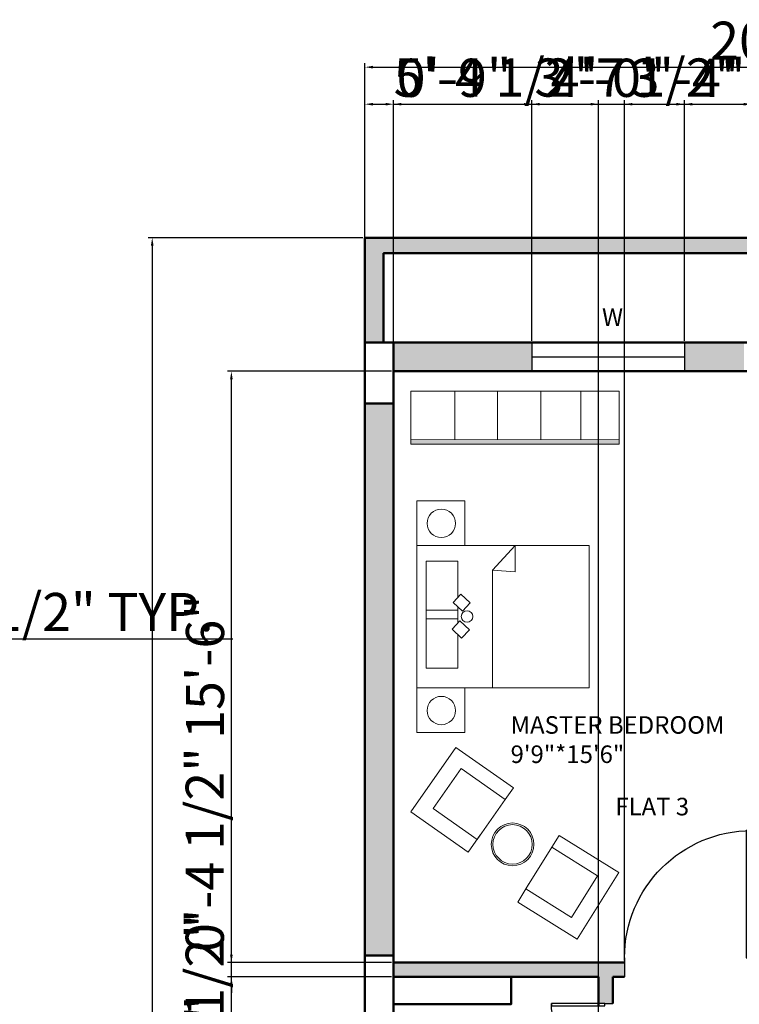
# Model space of a CAD drawing. Units: inches. Extents: x 2063 to 3370, y 2091 to 2971.
# Tile 9 of 14: x 2494 to 2721, y 2623 to 2933. Entities that reach past the tile are written whole.
import ezdxf

# ---------------------------------------------------------------- set-up
doc = ezdxf.new("R2010")
doc.units = ezdxf.units.IN
for name, color, linetype, lineweight in [('A-ANNO-DIMS', 2, 'Continuous', 18), ('A-ANNO-TEXT', 7, 'Continuous', 18), ('A-AREA-IDEN', 3, 'Continuous', 18), ('A-COLS', 7, 'Continuous', 50), ('A-DOOR', 4, 'Continuous', 25), ('A-FURN', 8, 'Continuous', 18), ('A-GLAZ', 131, 'Continuous', 25), ('A-WALL', 7, 'Continuous', 50), ('A-WALL-PATT', 8, 'Continuous', 13)]:
    doc.layers.add(name, color=color, linetype=linetype, lineweight=lineweight)
doc.styles.get("Standard").update_dxf_attribs({"font": 'arial.ttf'})
doc.dimstyles.new('ISO-25', dxfattribs={"dimtxt": 12, "dimasz": 2.5, "dimexe": 1.25, "dimexo": 0.625, "dimtad": 1, "dimdec": 0, "dimlunit": 4, "dimtxsty": 'Standard', "dimcen": 2.5, "dimadec": 0, "dimazin": 0, "dimtfac": 1, "dimtdec": 0, "dimtmove": 0, "dimatfit": 3, "dimfxl": 1, "dimarcsym": 0})

# ---------------------------------------------------------------- blocks, each defined once
blk = doc.blocks.new('*D7')
at = {"layer": 'A-ANNO-DIMS', "color": 0, "lineweight": -2, "transparency": 16777216}
for p, q in [((2602.75, 2865.05), (2602.75, 2919.33)), ((2605.25, 2918.08), (2840.25, 2918.08)), ((2842.75, 2865.05), (2842.75, 2919.33))]:
    blk.add_line(p, q, dxfattribs=at)
at = {"layer": 'A-ANNO-DIMS', "color": 0, "transparency": 16777216}
for points in [[(2605.25, 2918.5), (2605.25, 2917.67), (2602.75, 2918.08)], [(2840.25, 2918.5), (2840.25, 2917.67), (2842.75, 2918.08)]]:
    blk.add_solid(points, dxfattribs=at)
at = {"layer": 'Defpoints', "color": 0, "transparency": 16777216}
for p in [(2842.75, 2918.08), (2602.75, 2864.43), (2842.75, 2864.43)]:
    blk.add_point(p, dxfattribs=at)
at = {"layer": 'A-ANNO-DIMS', "color": 0, "transparency": 16777216, "insert": (2722.75, 2924.84), "char_height": 12, "attachment_point": 5}
blk.add_mtext("20'", dxfattribs=at)
blk = doc.blocks.new('*D8')
at = {"layer": 'A-ANNO-DIMS', "color": 0, "lineweight": -2, "transparency": 16777216}
for p, q in [((2602.12, 2864.43), (2534.59, 2864.43)), ((2535.84, 2861.93), (2535.84, 2146.93)), ((2602.12, 2144.43), (2534.59, 2144.43))]:
    blk.add_line(p, q, dxfattribs=at)
at = {"layer": 'A-ANNO-DIMS', "color": 0, "transparency": 16777216}
for points in [[(2535.42, 2861.93), (2536.25, 2861.93), (2535.84, 2864.43)], [(2535.42, 2146.93), (2536.25, 2146.93), (2535.84, 2144.43)]]:
    blk.add_solid(points, dxfattribs=at)
at = {"layer": 'Defpoints', "color": 0, "transparency": 16777216}
for p in [(2602.75, 2864.43), (2535.84, 2144.43), (2602.75, 2144.43)]:
    blk.add_point(p, dxfattribs=at)
at = {"layer": 'A-ANNO-DIMS', "color": 0, "transparency": 16777216, "insert": (2529.08, 2504.43), "char_height": 12, "attachment_point": 5, "rotation": 90}
blk.add_mtext("60'", dxfattribs=at)
blk = doc.blocks.new('*U2')
for p, q in [((0, 0), (0, -6)), ((40, 0), (40, -6))]:
    blk.add_line(p, q)
blk.add_lwpolyline([(0, 0), (0, 40), (1.75, 40), (1.75, 0)], close=True)
blk.add_arc((0, 0), 40, 0, 90)
blk = doc.blocks.new('BED-DOUBLE')
for p, q in [((23.79, 50.98), (30.96, 58.78)), ((30.96, 58.78), (30.96, 50.54)), ((23.79, 14), (23.79, 50.98)), ((30.96, 50.54), (23.79, 50.98))]:
    blk.add_line(p, q)
for points in [[(0, 58.78), (15.11, 58.78), (15.11, 72.78), (0, 72.78)], [(0, 58.78), (54.26, 58.78), (54.26, 14), (0, 14)], [(11.45, 40.86), (13.89, 43.46), (16.84, 40.71), (14.4, 38.1)], [(11.16, 32.43), (13.59, 35.03), (16.54, 32.28), (14.11, 29.67)], [(0, 0), (15.11, 0), (15.11, 14), (0, 14)]]:
    blk.add_lwpolyline(points, close=True)
for points in [[(12.88, 42.39), (12.88, 53.87), (2.9, 53.87), (2.9, 35.71), (12.88, 35.71), (12.88, 39.52)], [(12.88, 34.27), (12.88, 38.39), (2.9, 38.39), (2.9, 20.23), (12.88, 20.23), (12.88, 30.81)]]:
    blk.add_lwpolyline(points)
for centre, radius in [((7.71, 65.74), 4.47), ((15.81, 36.46), 1.81), ((7.71, 6.86), 4.47)]:
    blk.add_circle(centre, radius)
blk = doc.blocks.new('WARDROBE')
for p, q in [((13.88, 1.44), (13.88, 16.75)), ((27.33, 1.44), (27.33, 16.75)), ((40.97, 1.44), (40.97, 16.75)), ((53.56, 1.44), (53.56, 16.75)), ((0, 1.42), (65.55, 1.52))]:
    blk.add_line(p, q)
blk.add_lwpolyline([(0, 16.75), (65.55, 16.75), (65.55, 0), (0, 0)], close=True)
blk = doc.blocks.new('ARMCHAIR')
for p, q in [((10.7, 28.87), (13.03, 32.61)), ((13.03, 32.61), (31.78, 20.96)), ((31.78, 20.96), (18.75, 0)), ((0, 11.65), (3.54, 17.35)), ((18.75, 0), (0, 11.65))]:
    blk.add_line(p, q)
blk.add_lwpolyline([(2.55, 15.75), (16.92, 6.82), (25.07, 19.93), (10.7, 28.87)], close=True)
blk = doc.blocks.new('*D22')
at = {"layer": 'A-ANNO-DIMS', "color": 0, "lineweight": -2, "transparency": 16777216}
for p, q in [((2286.92, 2747.51), (2286.92, 2737.05)), ((2352.47, 2747.51), (2352.47, 2737.05)), ((2289.42, 2738.3), (2349.97, 2738.3)), ((2352.47, 2738.3), (2561.2, 2738.3))]:
    blk.add_line(p, q, dxfattribs=at)
at = {"layer": 'A-ANNO-DIMS', "color": 0, "transparency": 16777216}
for points in [[(2289.42, 2738.72), (2289.42, 2737.89), (2286.92, 2738.3)], [(2349.97, 2738.72), (2349.97, 2737.89), (2352.47, 2738.3)]]:
    blk.add_solid(points, dxfattribs=at)
at = {"layer": 'Defpoints', "color": 0, "transparency": 16777216}
for p in [(2286.92, 2748.13), (2352.47, 2748.13), (2352.47, 2738.3)]:
    blk.add_point(p, dxfattribs=at)
at = {"layer": 'A-ANNO-DIMS', "color": 0, "transparency": 16777216, "insert": (2458.09, 2745.14), "char_height": 12, "attachment_point": 5}
blk.add_mtext('WARDROBE 5\'-5 1/2" TYP.', dxfattribs=at)
blk = doc.blocks.new('*D79')
at = {"layer": 'A-ANNO-DIMS', "color": 0, "lineweight": -2, "transparency": 16777216}
for p, q in [((2602.75, 2832.05), (2602.75, 2907.68)), ((2605.25, 2906.43), (2609.25, 2906.43)), ((2611.75, 2823.05), (2611.75, 2907.68)), ((2611.75, 2906.43), (2647.4, 2906.43))]:
    blk.add_line(p, q, dxfattribs=at)
at = {"layer": 'A-ANNO-DIMS', "color": 0, "transparency": 16777216}
for points in [[(2605.25, 2906.84), (2605.25, 2906.01), (2602.75, 2906.43)], [(2609.25, 2906.84), (2609.25, 2906.01), (2611.75, 2906.43)]]:
    blk.add_solid(points, dxfattribs=at)
at = {"layer": 'Defpoints', "color": 0, "transparency": 16777216}
for p in [(2611.75, 2906.43), (2602.75, 2831.43), (2611.75, 2822.43)]:
    blk.add_point(p, dxfattribs=at)
at = {"layer": 'A-ANNO-DIMS', "color": 0, "transparency": 16777216, "insert": (2630.82, 2913.18), "char_height": 12, "attachment_point": 5}
blk.add_mtext('0\'-9"', dxfattribs=at)
blk = doc.blocks.new('*D80')
at = {"layer": 'A-ANNO-DIMS', "color": 0, "lineweight": -2, "transparency": 16777216}
for p, q in [((2611.75, 2823.05), (2611.75, 2907.68)), ((2614.25, 2906.43), (2652.77, 2906.43)), ((2655.27, 2832.05), (2655.27, 2907.68)), ((2655.27, 2906.43), (2718.87, 2906.43))]:
    blk.add_line(p, q, dxfattribs=at)
at = {"layer": 'A-ANNO-DIMS', "color": 0, "transparency": 16777216}
for points in [[(2614.25, 2906.84), (2614.25, 2906.01), (2611.75, 2906.43)], [(2652.77, 2906.84), (2652.77, 2906.01), (2655.27, 2906.43)]]:
    blk.add_solid(points, dxfattribs=at)
at = {"layer": 'Defpoints', "color": 0, "transparency": 16777216}
for p in [(2655.27, 2906.43), (2655.27, 2831.43), (2611.75, 2822.43)]:
    blk.add_point(p, dxfattribs=at)
at = {"layer": 'A-ANNO-DIMS', "color": 0, "transparency": 16777216, "insert": (2688.32, 2913.26), "char_height": 12, "attachment_point": 5}
blk.add_mtext('3\'-7 1/2"', dxfattribs=at)
blk = doc.blocks.new('*D81')
at = {"layer": 'A-ANNO-DIMS', "color": 0, "lineweight": -2, "transparency": 16777216}
for p, q in [((2655.27, 2832.05), (2655.27, 2907.68)), ((2657.77, 2906.43), (2700.77, 2906.43)), ((2703.27, 2832.05), (2703.27, 2907.68))]:
    blk.add_line(p, q, dxfattribs=at)
at = {"layer": 'A-ANNO-DIMS', "color": 0, "transparency": 16777216}
for points in [[(2657.77, 2906.84), (2657.77, 2906.01), (2655.27, 2906.43)], [(2700.77, 2906.84), (2700.77, 2906.01), (2703.27, 2906.43)]]:
    blk.add_solid(points, dxfattribs=at)
at = {"layer": 'Defpoints', "color": 0, "transparency": 16777216}
for p in [(2703.27, 2906.43), (2655.27, 2831.43), (2703.27, 2831.43)]:
    blk.add_point(p, dxfattribs=at)
at = {"layer": 'A-ANNO-DIMS', "color": 0, "transparency": 16777216, "insert": (2679.27, 2913.18), "char_height": 12, "attachment_point": 5}
blk.add_mtext('4\'-0"', dxfattribs=at)
blk = doc.blocks.new('*D82')
at = {"layer": 'A-ANNO-DIMS', "color": 0, "lineweight": -2, "transparency": 16777216}
for p, q in [((2703.27, 2832.05), (2703.27, 2907.68)), ((2705.77, 2906.43), (2726.25, 2906.43)), ((2728.75, 2823.05), (2728.75, 2907.68)), ((2728.75, 2906.43), (2792.56, 2906.43))]:
    blk.add_line(p, q, dxfattribs=at)
at = {"layer": 'A-ANNO-DIMS', "color": 0, "transparency": 16777216}
for points in [[(2705.77, 2906.84), (2705.77, 2906.01), (2703.27, 2906.43)], [(2726.25, 2906.84), (2726.25, 2906.01), (2728.75, 2906.43)]]:
    blk.add_solid(points, dxfattribs=at)
at = {"layer": 'Defpoints', "color": 0, "transparency": 16777216}
for p in [(2728.75, 2906.43), (2703.27, 2831.43), (2728.75, 2822.43)]:
    blk.add_point(p, dxfattribs=at)
at = {"layer": 'A-ANNO-DIMS', "color": 0, "transparency": 16777216, "insert": (2761.9, 2913.26), "char_height": 12, "attachment_point": 5}
blk.add_mtext('2\'-1 1/2"', dxfattribs=at)
blk = doc.blocks.new('*D97')
at = {"layer": 'A-ANNO-DIMS', "color": 0, "lineweight": -2, "transparency": 16777216}
for p, q in [((2611.75, 2584.55), (2611.75, 2907.68)), ((2614.25, 2906.43), (2673.75, 2906.43)), ((2676.25, 2584.55), (2676.25, 2907.68))]:
    blk.add_line(p, q, dxfattribs=at)
at = {"layer": 'A-ANNO-DIMS', "color": 0, "transparency": 16777216}
for points in [[(2614.25, 2906.84), (2614.25, 2906.01), (2611.75, 2906.43)], [(2673.75, 2906.84), (2673.75, 2906.01), (2676.25, 2906.43)]]:
    blk.add_solid(points, dxfattribs=at)
at = {"layer": 'Defpoints', "color": 0, "transparency": 16777216}
for p in [(2676.25, 2906.43), (2611.75, 2583.93), (2676.25, 2583.93)]:
    blk.add_point(p, dxfattribs=at)
at = {"layer": 'A-ANNO-DIMS', "color": 0, "transparency": 16777216, "insert": (2644, 2913.26), "char_height": 12, "attachment_point": 5}
blk.add_mtext('5\'-4 1/2"', dxfattribs=at)
blk = doc.blocks.new('*D107')
at = {"layer": 'A-ANNO-DIMS', "color": 0, "lineweight": -2, "transparency": 16777216}
for p, q in [((2560.75, 2586.43), (2560.75, 2650.04)), ((2611.12, 2583.93), (2559.5, 2583.93)), ((2560.75, 2579.43), (2560.75, 2583.93)), ((2611.12, 2579.43), (2559.5, 2579.43)), ((2560.75, 2576.93), (2560.75, 2574.43))]:
    blk.add_line(p, q, dxfattribs=at)
at = {"layer": 'A-ANNO-DIMS', "color": 0, "transparency": 16777216}
for points in [[(2560.33, 2586.43), (2561.16, 2586.43), (2560.75, 2583.93)], [(2560.33, 2576.93), (2561.16, 2576.93), (2560.75, 2579.43)]]:
    blk.add_solid(points, dxfattribs=at)
at = {"layer": 'Defpoints', "color": 0, "transparency": 16777216}
for p in [(2560.75, 2583.93), (2611.75, 2583.93), (2611.75, 2579.43)]:
    blk.add_point(p, dxfattribs=at)
at = {"layer": 'A-ANNO-DIMS', "color": 0, "transparency": 16777216, "insert": (2553.92, 2619.48), "char_height": 12, "attachment_point": 5, "rotation": 90}
blk.add_mtext('0\'-4 1/2"', dxfattribs=at)
blk = doc.blocks.new('*D108')
at = {"layer": 'A-ANNO-DIMS', "color": 0, "lineweight": -2, "transparency": 16777216}
for p, q in [((2611.12, 2631.93), (2559.5, 2631.93)), ((2560.75, 2586.43), (2560.75, 2629.43)), ((2611.12, 2583.93), (2559.5, 2583.93))]:
    blk.add_line(p, q, dxfattribs=at)
at = {"layer": 'A-ANNO-DIMS', "color": 0, "transparency": 16777216}
for points in [[(2560.33, 2629.43), (2561.16, 2629.43), (2560.75, 2631.93)], [(2560.33, 2586.43), (2561.16, 2586.43), (2560.75, 2583.93)]]:
    blk.add_solid(points, dxfattribs=at)
at = {"layer": 'Defpoints', "color": 0, "transparency": 16777216}
for p in [(2560.75, 2631.93), (2611.75, 2631.93), (2611.75, 2583.93)]:
    blk.add_point(p, dxfattribs=at)
at = {"layer": 'A-ANNO-DIMS', "color": 0, "transparency": 16777216, "insert": (2554, 2607.93), "char_height": 12, "attachment_point": 5, "rotation": 90}
blk.add_mtext('4\'-0"', dxfattribs=at)
blk = doc.blocks.new('*D109')
at = {"layer": 'A-ANNO-DIMS', "color": 0, "lineweight": -2, "transparency": 16777216}
for p, q in [((2560.75, 2638.93), (2560.75, 2702.54)), ((2611.12, 2636.43), (2559.5, 2636.43)), ((2560.75, 2631.93), (2560.75, 2636.43)), ((2611.12, 2631.93), (2559.5, 2631.93)), ((2560.75, 2629.43), (2560.75, 2626.93))]:
    blk.add_line(p, q, dxfattribs=at)
at = {"layer": 'A-ANNO-DIMS', "color": 0, "transparency": 16777216}
for points in [[(2560.33, 2638.93), (2561.16, 2638.93), (2560.75, 2636.43)], [(2560.33, 2629.43), (2561.16, 2629.43), (2560.75, 2631.93)]]:
    blk.add_solid(points, dxfattribs=at)
at = {"layer": 'Defpoints', "color": 0, "transparency": 16777216}
for p in [(2560.75, 2636.43), (2611.75, 2636.43), (2611.75, 2631.93)]:
    blk.add_point(p, dxfattribs=at)
at = {"layer": 'A-ANNO-DIMS', "color": 0, "transparency": 16777216, "insert": (2553.92, 2671.98), "char_height": 12, "attachment_point": 5, "rotation": 90}
blk.add_mtext('0\'-4 1/2"', dxfattribs=at)
blk = doc.blocks.new('*D110')
at = {"layer": 'A-ANNO-DIMS', "color": 0, "lineweight": -2, "transparency": 16777216}
for p, q in [((2611.12, 2822.43), (2559.5, 2822.43)), ((2560.75, 2638.93), (2560.75, 2819.93)), ((2611.12, 2636.43), (2559.5, 2636.43))]:
    blk.add_line(p, q, dxfattribs=at)
at = {"layer": 'A-ANNO-DIMS', "color": 0, "transparency": 16777216}
for points in [[(2560.33, 2819.93), (2561.16, 2819.93), (2560.75, 2822.43)], [(2560.33, 2638.93), (2561.16, 2638.93), (2560.75, 2636.43)]]:
    blk.add_solid(points, dxfattribs=at)
at = {"layer": 'Defpoints', "color": 0, "transparency": 16777216}
for p in [(2560.75, 2822.43), (2611.75, 2822.43), (2611.75, 2636.43)]:
    blk.add_point(p, dxfattribs=at)
at = {"layer": 'A-ANNO-DIMS', "color": 0, "transparency": 16777216, "insert": (2554, 2729.43), "char_height": 12, "attachment_point": 5, "rotation": 90}
blk.add_mtext('15\'-6"', dxfattribs=at)
blk = doc.blocks.new('*D128')
at = {"layer": 'A-ANNO-DIMS', "color": 0, "lineweight": -2, "transparency": 16777216}
for p, q in [((2684.44, 2637.05), (2684.44, 2907.68)), ((2686.94, 2906.43), (2721.94, 2906.43)), ((2724.44, 2632.55), (2724.44, 2907.68))]:
    blk.add_line(p, q, dxfattribs=at)
at = {"layer": 'A-ANNO-DIMS', "color": 0, "transparency": 16777216}
for points in [[(2686.94, 2906.84), (2686.94, 2906.01), (2684.44, 2906.43)], [(2721.94, 2906.84), (2721.94, 2906.01), (2724.44, 2906.43)]]:
    blk.add_solid(points, dxfattribs=at)
at = {"layer": 'Defpoints', "color": 0, "transparency": 16777216}
for p in [(2724.44, 2906.43), (2684.44, 2636.43), (2724.44, 2631.93)]:
    blk.add_point(p, dxfattribs=at)
at = {"layer": 'A-ANNO-DIMS', "color": 0, "transparency": 16777216, "insert": (2704.44, 2913.18), "char_height": 12, "attachment_point": 5}
blk.add_mtext('3\'-4"', dxfattribs=at)

msp = doc.modelspace()

# ---------------------------------------------------------------- hatches: boundary and pattern name
at = {"layer": 'A-FURN'}
h = msp.add_hatch(color=256, dxfattribs=at)
h.dxf.hatch_style = 1
h.paths.add_polyline_path([(2682.71, 2800.98), (2617.16, 2800.89), (2617.16, 2799.47), (2682.71, 2799.47)])
at = {"layer": 'A-WALL-PATT'}
h = msp.add_hatch(color=256, dxfattribs=at)
h.dxf.hatch_style = 1
h.paths.add_polyline_path([(2842.75, 2864.43), (2602.75, 2864.43), (2602.75, 2831.43), (2608.62, 2831.43), (2608.62, 2859.54), (2836.36, 2859.54), (2836.36, 2831.15), (2842.75, 2831.15)])
h.paths.add_polyline_path([(2775.49, 2177.04), (2815.13, 2177.04), (2815.13, 2197.65), (2775.49, 2197.65)], flags=9)
h.paths.add_polyline_path([(2634.18, 2285.75), (2670.81, 2285.75), (2670.81, 2306.35), (2634.18, 2306.35)], flags=9)
h.paths.add_polyline_path([(2701.65, 2293.1), (2755.85, 2293.1), (2755.85, 2313.71), (2701.65, 2313.71)], flags=9)
h.paths.add_polyline_path([(2735.8, 2415.55), (2772.95, 2415.55), (2772.95, 2436.13), (2735.8, 2436.13)], flags=9)
h.paths.add_polyline_path([(2641.75, 2422.21), (2718.67, 2422.21), (2718.67, 2442.82), (2641.75, 2442.82)], flags=9)
h.paths.add_polyline_path([(2710.43, 2552.92), (2764.91, 2552.92), (2764.91, 2573.53), (2710.43, 2573.53)], flags=9)
h.paths.add_polyline_path([(2625.23, 2527.83), (2661.86, 2527.83), (2661.86, 2548.44), (2625.23, 2548.44)], flags=9)
h.paths.add_polyline_path([(2627.53, 2598.16), (2652.13, 2598.16), (2652.13, 2618.77), (2627.53, 2618.77)], flags=9)
h.paths.add_polyline_path([(2646.64, 2696.08), (2723.56, 2696.08), (2723.56, 2716.69), (2646.64, 2716.69)], flags=9)
h.paths.add_polyline_path([(2791.65, 2795.64), (2828.72, 2795.64), (2828.72, 2807.02), (2791.65, 2807.02)], flags=9)
h.paths.add_polyline_path([(2751.88, 2214.78), (2761.93, 2214.78), (2761.93, 2226.17), (2751.88, 2226.17)], flags=9)
h.paths.add_polyline_path([(2664.96, 2215.71), (2675, 2215.71), (2675, 2227.09), (2664.96, 2227.09)], flags=9)
h.paths.add_polyline_path([(2788.26, 2413.43), (2796.17, 2413.43), (2796.17, 2424.82), (2788.26, 2424.82)], flags=9)
h.paths.add_polyline_path([(2728.86, 2795.64), (2765.93, 2795.64), (2765.93, 2807.02), (2728.86, 2807.02)], flags=9)
h.paths.add_polyline_path([(2760.39, 2726.09), (2823.16, 2726.09), (2823.16, 2746.7), (2760.39, 2746.7)], flags=9)
h = msp.add_hatch(color=256, dxfattribs=at)
h.dxf.hatch_style = 1
h.paths.add_polyline_path([(2290.22, 2192.43), (2278.22, 2192.43), (2182.22, 2192.43), (2182.22, 2189.43), (2182.22, 2187.43), (2278.22, 2187.43), (2290.22, 2187.42)])
h.paths.add_polyline_path([(2748.25, 2192.43), (2736.25, 2192.43), (2640.25, 2192.43), (2640.25, 2189.43), (2640.25, 2187.43), (2736.25, 2187.43), (2748.25, 2187.42)], flags=17)
h.paths.add_polyline_path([(2653.66, 2234.43), (2611.75, 2234.43), (2611.75, 2232.93), (2611.75, 2225.43), (2653.66, 2225.43)])
h.paths.add_polyline_path([(2717.13, 2234.43), (2675.81, 2234.43), (2675.81, 2225.43), (2717.13, 2225.43)])
h.paths.add_polyline_path([(2611.75, 2222.57), (2602.75, 2222.57), (2602.75, 2144.43), (2842.75, 2144.43), (2842.75, 2220.3), (2833.75, 2220.3), (2833.75, 2153.43), (2829.39, 2153.43), (2754.78, 2153.43), (2611.75, 2153.43)])
h.paths.add_polyline_path([(2687.64, 2308.91), (2683.14, 2308.91), (2683.14, 2234.43), (2687.64, 2234.43)])
h.paths.add_polyline_path([(2744.5, 2234.43), (2736.25, 2234.43), (2736.25, 2225.43), (2744.5, 2225.43)])
h.paths.add_polyline_path([(2785.14, 2260.02), (2782.31, 2260.02), (2780.64, 2260.02), (2780.64, 2234.43), (2766.65, 2234.43), (2766.65, 2225.43), (2785.14, 2225.43)])
h.paths.add_polyline_path([(2842.75, 2363.93), (2833.75, 2363.93), (2833.75, 2239.41), (2842.75, 2239.41)])
h.paths.add_polyline_path([(2775.49, 2177.04), (2815.13, 2177.04), (2815.13, 2197.65), (2775.49, 2197.65)], flags=25)
h.paths.add_polyline_path([(2634.18, 2285.75), (2670.81, 2285.75), (2670.81, 2306.35), (2634.18, 2306.35)], flags=9)
h.paths.add_polyline_path([(2701.65, 2293.1), (2755.85, 2293.1), (2755.85, 2313.71), (2701.65, 2313.71)], flags=9)
h.paths.add_polyline_path([(2735.8, 2415.55), (2772.95, 2415.55), (2772.95, 2436.13), (2735.8, 2436.13)], flags=9)
h.paths.add_polyline_path([(2641.75, 2422.21), (2718.67, 2422.21), (2718.67, 2442.82), (2641.75, 2442.82)], flags=9)
h.paths.add_polyline_path([(2710.43, 2552.92), (2764.91, 2552.92), (2764.91, 2573.53), (2710.43, 2573.53)], flags=9)
h.paths.add_polyline_path([(2625.23, 2527.83), (2661.86, 2527.83), (2661.86, 2548.44), (2625.23, 2548.44)], flags=9)
h.paths.add_polyline_path([(2627.53, 2598.16), (2652.13, 2598.16), (2652.13, 2618.77), (2627.53, 2618.77)], flags=9)
h.paths.add_polyline_path([(2646.64, 2696.08), (2723.56, 2696.08), (2723.56, 2716.69), (2646.64, 2716.69)], flags=9)
h.paths.add_polyline_path([(2791.65, 2795.64), (2828.72, 2795.64), (2828.72, 2807.02), (2791.65, 2807.02)], flags=9)
h.paths.add_polyline_path([(2751.88, 2214.78), (2761.93, 2214.78), (2761.93, 2226.17), (2751.88, 2226.17)], flags=9)
h.paths.add_polyline_path([(2788.26, 2413.43), (2796.17, 2413.43), (2796.17, 2424.82), (2788.26, 2424.82)], flags=9)
h.paths.add_polyline_path([(2761.97, 2835.24), (2769.88, 2835.24), (2769.88, 2846.62), (2761.97, 2846.62)], flags=9)
h.paths.add_polyline_path([(2675.89, 2833.68), (2685.93, 2833.68), (2685.93, 2845.06), (2675.89, 2845.06)], flags=9)
h.paths.add_polyline_path([(2728.86, 2795.64), (2765.93, 2795.64), (2765.93, 2807.02), (2728.86, 2807.02)], flags=9)
h.paths.add_polyline_path([(2760.39, 2726.09), (2823.16, 2726.09), (2823.16, 2746.7), (2760.39, 2746.7)], flags=9)
h = msp.add_hatch(color=256, dxfattribs=at)
h.dxf.hatch_style = 1
h.paths.add_polyline_path([(2680.75, 2631.93), (2684.44, 2631.93), (2684.44, 2636.43), (2683.1, 2636.43), (2611.75, 2636.43), (2611.75, 2631.93), (2648.72, 2631.93), (2671.75, 2631.93), (2676.25, 2631.93), (2676.25, 2623.58), (2678.23, 2623.58), (2680.75, 2623.58)])
h.paths.add_polyline_path([(2728.75, 2636.43), (2724.44, 2636.43), (2724.44, 2631.93), (2728.75, 2631.93)])
h.paths.add_polyline_path([(2772.02, 2636.43), (2733.25, 2636.43), (2733.25, 2631.93), (2772.02, 2631.93)])
h.paths.add_polyline_path([(2733.25, 2636.43), (2728.75, 2636.43), (2728.75, 2631.93), (2733.25, 2631.93)])
h.paths.add_polyline_path([(2833.75, 2636.43), (2812.02, 2636.43), (2812.02, 2631.93), (2833.75, 2631.93)])
h.paths.add_polyline_path([(2842.75, 2626.16), (2833.75, 2626.16), (2833.75, 2585.28), (2842.75, 2585.28)])
h.paths.add_polyline_path([(2842.75, 2679.03), (2833.75, 2679.03), (2833.75, 2645.28), (2842.75, 2645.28)])
h.paths.add_polyline_path([(2611.75, 2619.52), (2602.75, 2619.52), (2602.75, 2548.5), (2611.75, 2548.5), (2611.75, 2579.43)])
h.paths.add_polyline_path([(2646.64, 2696.08), (2723.56, 2696.08), (2723.56, 2716.69), (2646.64, 2716.69)], flags=9)
h.paths.add_polyline_path([(2791.65, 2795.64), (2828.72, 2795.64), (2828.72, 2807.02), (2791.65, 2807.02)], flags=9)
h.paths.add_polyline_path([(2761.97, 2835.24), (2769.88, 2835.24), (2769.88, 2846.62), (2761.97, 2846.62)], flags=9)
h.paths.add_polyline_path([(2675.89, 2833.68), (2685.93, 2833.68), (2685.93, 2845.06), (2675.89, 2845.06)], flags=9)
h.paths.add_polyline_path([(2728.86, 2795.64), (2765.93, 2795.64), (2765.93, 2807.02), (2728.86, 2807.02)], flags=9)
h.paths.add_polyline_path([(2775.49, 2177.04), (2815.13, 2177.04), (2815.13, 2197.65), (2775.49, 2197.65)], flags=9)
h.paths.add_polyline_path([(2634.18, 2285.75), (2670.81, 2285.75), (2670.81, 2306.35), (2634.18, 2306.35)], flags=9)
h.paths.add_polyline_path([(2701.65, 2293.1), (2755.85, 2293.1), (2755.85, 2313.71), (2701.65, 2313.71)], flags=9)
h.paths.add_polyline_path([(2735.8, 2415.55), (2772.95, 2415.55), (2772.95, 2436.13), (2735.8, 2436.13)], flags=9)
h.paths.add_polyline_path([(2641.75, 2422.21), (2718.67, 2422.21), (2718.67, 2442.82), (2641.75, 2442.82)], flags=9)
h.paths.add_polyline_path([(2710.43, 2552.92), (2764.91, 2552.92), (2764.91, 2573.53), (2710.43, 2573.53)], flags=9)
h.paths.add_polyline_path([(2625.23, 2527.83), (2661.86, 2527.83), (2661.86, 2548.44), (2625.23, 2548.44)], flags=9)
h.paths.add_polyline_path([(2751.88, 2214.78), (2761.93, 2214.78), (2761.93, 2226.17), (2751.88, 2226.17)], flags=9)
h.paths.add_polyline_path([(2664.96, 2215.71), (2675, 2215.71), (2675, 2227.09), (2664.96, 2227.09)], flags=9)
h.paths.add_polyline_path([(2788.26, 2413.43), (2796.17, 2413.43), (2796.17, 2424.82), (2788.26, 2424.82)], flags=9)
h = msp.add_hatch(color=256, dxfattribs=at)
h.dxf.hatch_style = 1
h.paths.add_polyline_path([(2611.75, 2343.93), (2611.75, 2477.43), (2611.75, 2514.15), (2602.75, 2514.15), (2602.75, 2241.68), (2611.75, 2241.68), (2611.75, 2258.43)])
h.paths.add_polyline_path([(2775.49, 2177.04), (2815.13, 2177.04), (2815.13, 2197.65), (2775.49, 2197.65)], flags=9)
h.paths.add_polyline_path([(2735.8, 2415.55), (2772.95, 2415.55), (2772.95, 2436.13), (2735.8, 2436.13)], flags=9)
h.paths.add_polyline_path([(2641.75, 2422.21), (2718.67, 2422.21), (2718.67, 2442.82), (2641.75, 2442.82)], flags=9)
h.paths.add_polyline_path([(2710.43, 2552.92), (2764.91, 2552.92), (2764.91, 2573.53), (2710.43, 2573.53)], flags=9)
h.paths.add_polyline_path([(2625.23, 2527.83), (2661.86, 2527.83), (2661.86, 2548.44), (2625.23, 2548.44)], flags=9)
h.paths.add_polyline_path([(2627.53, 2598.16), (2652.13, 2598.16), (2652.13, 2618.77), (2627.53, 2618.77)], flags=9)
h.paths.add_polyline_path([(2646.64, 2696.08), (2723.56, 2696.08), (2723.56, 2716.69), (2646.64, 2716.69)], flags=9)
h.paths.add_polyline_path([(2791.65, 2795.64), (2828.72, 2795.64), (2828.72, 2807.02), (2791.65, 2807.02)], flags=9)
h.paths.add_polyline_path([(2751.88, 2214.78), (2761.93, 2214.78), (2761.93, 2226.17), (2751.88, 2226.17)], flags=9)
h.paths.add_polyline_path([(2788.26, 2413.43), (2796.17, 2413.43), (2796.17, 2424.82), (2788.26, 2424.82)], flags=9)
h.paths.add_polyline_path([(2761.97, 2835.24), (2769.88, 2835.24), (2769.88, 2846.62), (2761.97, 2846.62)], flags=9)
h.paths.add_polyline_path([(2675.89, 2833.68), (2685.93, 2833.68), (2685.93, 2845.06), (2675.89, 2845.06)], flags=9)
h.paths.add_polyline_path([(2728.86, 2795.64), (2765.93, 2795.64), (2765.93, 2807.02), (2728.86, 2807.02)], flags=9)
h.paths.add_polyline_path([(2760.39, 2726.09), (2823.16, 2726.09), (2823.16, 2746.7), (2760.39, 2746.7)], flags=9)
h = msp.add_hatch(color=256, dxfattribs=at)
h.dxf.hatch_style = 1
h.paths.add_polyline_path([(2785.14, 2468.43), (2780.64, 2468.43), (2780.64, 2429.31), (2785.14, 2429.31)])
h.paths.add_polyline_path([(2842.75, 2525.28), (2833.75, 2525.28), (2833.75, 2523.93), (2833.75, 2466.93), (2833.75, 2383.04), (2842.75, 2383.04)])
h.paths.add_polyline_path([(2789.73, 2477.43), (2680.75, 2477.43), (2680.75, 2579.43), (2680.75, 2589.96), (2678.23, 2589.96), (2676.25, 2589.96), (2676.25, 2583.93), (2667.25, 2583.93), (2611.75, 2583.93), (2611.75, 2579.43), (2671.75, 2579.43), (2676.25, 2579.43), (2676.25, 2477.43), (2611.75, 2477.43), (2611.75, 2468.43), (2728.75, 2468.43), (2789.73, 2468.43), (2789.73, 2471.41)])
h.paths.add_polyline_path([(2710.43, 2552.92), (2764.91, 2552.92), (2764.91, 2573.53), (2710.43, 2573.53)], flags=25)
h.paths.add_polyline_path([(2625.23, 2527.83), (2661.86, 2527.83), (2661.86, 2548.44), (2625.23, 2548.44)], flags=25)
h.paths.add_polyline_path([(2627.53, 2598.16), (2652.13, 2598.16), (2652.13, 2618.77), (2627.53, 2618.77)], flags=9)
h.paths.add_polyline_path([(2646.64, 2696.08), (2723.56, 2696.08), (2723.56, 2716.69), (2646.64, 2716.69)], flags=9)
h.paths.add_polyline_path([(2791.65, 2795.64), (2828.72, 2795.64), (2828.72, 2807.02), (2791.65, 2807.02)], flags=9)
h.paths.add_polyline_path([(2761.97, 2835.24), (2769.88, 2835.24), (2769.88, 2846.62), (2761.97, 2846.62)], flags=9)
h.paths.add_polyline_path([(2675.89, 2833.68), (2685.93, 2833.68), (2685.93, 2845.06), (2675.89, 2845.06)], flags=9)
h.paths.add_polyline_path([(2728.86, 2795.64), (2765.93, 2795.64), (2765.93, 2807.02), (2728.86, 2807.02)], flags=9)
h.paths.add_polyline_path([(2760.39, 2726.09), (2823.16, 2726.09), (2823.16, 2746.7), (2760.39, 2746.7)], flags=9)
h.paths.add_polyline_path([(2775.49, 2177.04), (2815.13, 2177.04), (2815.13, 2197.65), (2775.49, 2197.65)], flags=9)
h.paths.add_polyline_path([(2634.18, 2285.75), (2670.81, 2285.75), (2670.81, 2306.35), (2634.18, 2306.35)], flags=9)
h.paths.add_polyline_path([(2701.65, 2293.1), (2755.85, 2293.1), (2755.85, 2313.71), (2701.65, 2313.71)], flags=9)
h.paths.add_polyline_path([(2641.75, 2422.21), (2718.67, 2422.21), (2718.67, 2442.82), (2641.75, 2442.82)], flags=9)
h.paths.add_polyline_path([(2751.88, 2214.78), (2761.93, 2214.78), (2761.93, 2226.17), (2751.88, 2226.17)], flags=9)
h.paths.add_polyline_path([(2664.96, 2215.71), (2675, 2215.71), (2675, 2227.09), (2664.96, 2227.09)], flags=9)
h.paths.add_polyline_path([(2788.26, 2413.43), (2796.17, 2413.43), (2796.17, 2424.82), (2788.26, 2424.82)], flags=9)
h = msp.add_hatch(color=256, dxfattribs=at)
h.dxf.hatch_style = 1
h.paths.add_polyline_path([(2785.14, 2343.93), (2785.14, 2392.49), (2785.14, 2413.72), (2780.64, 2413.72), (2780.64, 2384.43), (2780.64, 2348.43), (2732.64, 2348.43), (2732.64, 2360.22), (2728.14, 2360.22), (2728.14, 2348.43), (2725.61, 2348.43), (2725.61, 2348.17), (2725.61, 2343.93), (2780.64, 2343.93), (2780.64, 2329.91), (2780.64, 2297.78), (2782.31, 2297.78), (2785.14, 2297.78)])
h.paths.add_polyline_path([(2732.64, 2396.29), (2731.36, 2396.29), (2728.14, 2396.29), (2728.14, 2379.34), (2732.64, 2379.34)], flags=17)
h.paths.add_polyline_path([(2732.64, 2468.43), (2728.14, 2468.43), (2728.14, 2417.8), (2731.36, 2417.8, -0.014809), (2732.64, 2417.76)])
h.paths.add_polyline_path([(2697.29, 2348.43), (2611.75, 2348.43), (2611.75, 2343.93), (2683.14, 2343.93), (2697.29, 2343.93)])
h.paths.add_polyline_path([(2710.43, 2552.92), (2764.91, 2552.92), (2764.91, 2573.53), (2710.43, 2573.53)], flags=9)
h.paths.add_polyline_path([(2625.23, 2527.83), (2661.86, 2527.83), (2661.86, 2548.44), (2625.23, 2548.44)], flags=9)
h.paths.add_polyline_path([(2627.53, 2598.16), (2652.13, 2598.16), (2652.13, 2618.77), (2627.53, 2618.77)], flags=9)
h.paths.add_polyline_path([(2646.64, 2696.08), (2723.56, 2696.08), (2723.56, 2716.69), (2646.64, 2716.69)], flags=9)
h.paths.add_polyline_path([(2791.65, 2795.64), (2828.72, 2795.64), (2828.72, 2807.02), (2791.65, 2807.02)], flags=9)
h.paths.add_polyline_path([(2761.97, 2835.24), (2769.88, 2835.24), (2769.88, 2846.62), (2761.97, 2846.62)], flags=9)
h.paths.add_polyline_path([(2675.89, 2833.68), (2685.93, 2833.68), (2685.93, 2845.06), (2675.89, 2845.06)], flags=9)
h.paths.add_polyline_path([(2728.86, 2795.64), (2765.93, 2795.64), (2765.93, 2807.02), (2728.86, 2807.02)], flags=9)
h.paths.add_polyline_path([(2760.39, 2726.09), (2823.16, 2726.09), (2823.16, 2746.7), (2760.39, 2746.7)], flags=9)
h = msp.add_hatch(color=256, dxfattribs=at)
h.dxf.hatch_style = 1
h.paths.add_polyline_path([(2655.27, 2831.43), (2611.75, 2831.43), (2611.75, 2822.43), (2655.27, 2822.43)])
h.paths.add_polyline_path([(2722.06, 2831.43), (2703.27, 2831.43), (2703.27, 2822.43), (2722.06, 2822.43)])
h.paths.add_polyline_path([(2754.66, 2831.43), (2741.18, 2831.43), (2741.18, 2822.43), (2754.66, 2822.43)])
h.paths.add_polyline_path([(2833.75, 2831.43), (2779.09, 2831.43), (2779.09, 2822.43), (2833.75, 2822.43)])
h.paths.add_polyline_path([(2790.07, 2822.43), (2785.57, 2822.43), (2785.57, 2774.43), (2790.07, 2774.43)])
h.paths.add_polyline_path([(2775.49, 2177.04), (2815.13, 2177.04), (2815.13, 2197.65), (2775.49, 2197.65)], flags=9)
h.paths.add_polyline_path([(2634.18, 2285.75), (2670.81, 2285.75), (2670.81, 2306.35), (2634.18, 2306.35)], flags=9)
h.paths.add_polyline_path([(2701.65, 2293.1), (2755.85, 2293.1), (2755.85, 2313.71), (2701.65, 2313.71)], flags=9)
h.paths.add_polyline_path([(2735.8, 2415.55), (2772.95, 2415.55), (2772.95, 2436.13), (2735.8, 2436.13)], flags=9)
h.paths.add_polyline_path([(2641.75, 2422.21), (2718.67, 2422.21), (2718.67, 2442.82), (2641.75, 2442.82)], flags=9)
h.paths.add_polyline_path([(2710.43, 2552.92), (2764.91, 2552.92), (2764.91, 2573.53), (2710.43, 2573.53)], flags=9)
h.paths.add_polyline_path([(2625.23, 2527.83), (2661.86, 2527.83), (2661.86, 2548.44), (2625.23, 2548.44)], flags=9)
h.paths.add_polyline_path([(2627.53, 2598.16), (2652.13, 2598.16), (2652.13, 2618.77), (2627.53, 2618.77)], flags=9)
h.paths.add_polyline_path([(2646.64, 2696.08), (2723.56, 2696.08), (2723.56, 2716.69), (2646.64, 2716.69)], flags=9)
h.paths.add_polyline_path([(2791.65, 2795.64), (2828.72, 2795.64), (2828.72, 2807.02), (2791.65, 2807.02)], flags=9)
h.paths.add_polyline_path([(2751.88, 2214.78), (2761.93, 2214.78), (2761.93, 2226.17), (2751.88, 2226.17)], flags=9)
h.paths.add_polyline_path([(2664.96, 2215.71), (2675, 2215.71), (2675, 2227.09), (2664.96, 2227.09)], flags=9)
h.paths.add_polyline_path([(2788.26, 2413.43), (2796.17, 2413.43), (2796.17, 2424.82), (2788.26, 2424.82)], flags=9)
h.paths.add_polyline_path([(2728.86, 2795.64), (2765.93, 2795.64), (2765.93, 2807.02), (2728.86, 2807.02)], flags=9)
h.paths.add_polyline_path([(2760.39, 2726.09), (2823.16, 2726.09), (2823.16, 2746.7), (2760.39, 2746.7)], flags=9)
h = msp.add_hatch(color=256, dxfattribs=at)
h.dxf.hatch_style = 1
h.paths.add_polyline_path([(2611.75, 2812.31), (2602.75, 2812.31), (2602.75, 2638.63), (2611.75, 2638.63)])

# ---------------------------------------------------------------- linework, layer by layer
at = {"layer": 'A-COLS'}
for points in [[(2602.75, 2831.43), (2611.75, 2831.43), (2611.75, 2812.31), (2602.75, 2812.31)], [(2602.75, 2638.63), (2611.75, 2638.63), (2611.75, 2619.52), (2602.75, 2619.52)]]:
    msp.add_lwpolyline(points, close=True, dxfattribs=at)
at = {"layer": 'A-FURN'}
for radius in [6.72, 6.2]:
    msp.add_circle((2649.23, 2673.62), radius, dxfattribs=at)
at = {"layer": 'A-GLAZ'}
for p, q in [((2655.27, 2831.43), (2655.27, 2822.43)), ((2703.27, 2831.43), (2703.27, 2822.43)), ((2655.27, 2826.93), (2703.27, 2826.93))]:
    msp.add_line(p, q, dxfattribs=at)
at = {"layer": 'A-WALL'}
for p, q in [((2611.75, 2822.43), (2728.75, 2822.43)), ((2611.75, 2822.43), (2728.75, 2822.43)), ((2611.75, 2636.43), (2683.1, 2636.43)), ((2683.1, 2636.43), (2684.44, 2636.43)), ((2611.75, 2631.93), (2671.75, 2631.93)), ((2611.75, 2631.93), (2671.75, 2631.93)), ((2671.75, 2631.93), (2676.25, 2631.93)), ((2676.25, 2622.85), (2676.25, 2631.93)), ((2680.75, 2631.93), (2683.1, 2631.93)), ((2680.75, 2631.93), (2684.44, 2631.93)), ((2680.75, 2623.58), (2680.75, 2631.93))]:
    msp.add_line(p, q, dxfattribs=at)
for points in [[(2602.75, 2144.43), (2842.75, 2144.43), (2842.75, 2864.43), (2602.75, 2864.43)], [(2836.36, 2831.43), (2836.36, 2859.54), (2608.62, 2859.54), (2608.62, 2831.43)], [(2611.75, 2631.93), (2648.72, 2631.93), (2648.72, 2623.33), (2611.75, 2623.33)]]:
    msp.add_lwpolyline(points, close=True, dxfattribs=at)
for points in [[(2611.75, 2822.43), (2611.75, 2576.43)], [(2611.75, 2631.93), (2611.75, 2583.93)]]:
    msp.add_lwpolyline(points, dxfattribs=at)

# ---------------------------------------------------------------- block references
at = {"layer": 'A-DOOR', "xscale": -1}
msp.add_blockref('*U2', (2724.44, 2637.93), dxfattribs=at)
at = {"layer": 'A-DOOR', "xscale": -0.4203428619043682, "yscale": 0.4203428619043682, "zscale": 0.4203428619043682, "rotation": 90}
msp.add_blockref('*U2', (2678.23, 2623.58), dxfattribs=at)
at = {"layer": 'A-FURN'}
for name, p in [('WARDROBE', (2617.16, 2799.47)), ('BED-DOUBLE', (2619.08, 2708.85)), ('ARMCHAIR', (2650.82, 2643.83))]:
    msp.add_blockref(name, p, dxfattribs=at)
at = {"layer": 'A-FURN', "extrusion": (0, 0, -1), "zscale": -1, "rotation": 66.95512356980076}
msp.add_blockref('ARMCHAIR', (-2624.55, 2666.62), dxfattribs=at)

# ---------------------------------------------------------------- texts
at = {"layer": 'A-ANNO-TEXT', "attachment_point": 1}
for s, heights, insert, char_height in [('W', [0], (2677.36, 2842.22), 5.52), ('FLAT 3', [14.84], (2681.55, 2688.26), 5.523)]:
    msp.add_mtext_dynamic_manual_height_columns(s, width=106.0361, gutter_width=27.61, heights=heights, dxfattribs=dict(at, insert=insert, char_height=char_height))
at = {"layer": 'A-AREA-IDEN', "insert": (2648.59, 2713.94), "char_height": 5.5229, "attachment_point": 1}
msp.add_mtext_dynamic_manual_height_columns('MASTER BEDROOM\\P9\'9"*15\'6"', width=106.0361, gutter_width=27.61, heights=[0], dxfattribs=at)

# ---------------------------------------------------------------- dimensions: what is measured, and where the dimension line sits
at = {"layer": 'A-ANNO-DIMS'}
for base, p1, p2, override, picture, middle in [((2842.75, 2918.08), (2602.75, 2864.43), (2842.75, 2864.43), {"dimclrd": 0, "dimclre": 0, "dimclrt": 0}, '*D7', (2722.75, 2924.84)), ((2655.27, 2906.43), (2611.75, 2822.43), (2655.27, 2831.43), {"dimdec": 1, "dimlfac": 1, "dimrnd": 0, "dimzin": 1, "dimdsep": 46, "dimlunit": 4, "dimfrac": 2}, '*D80', (2688.32, 2913.26)), ((2676.25, 2906.43), (2611.75, 2583.93), (2676.25, 2583.93), {"dimdec": 1, "dimlfac": 1, "dimrnd": 0, "dimzin": 1, "dimdsep": 46, "dimlunit": 4, "dimfrac": 2}, '*D97', (2644, 2913.26)), ((2728.75, 2906.43), (2703.27, 2831.43), (2728.75, 2822.43), {"dimdec": 1, "dimlfac": 1, "dimrnd": 0, "dimzin": 1, "dimdsep": 46, "dimlunit": 4, "dimfrac": 2}, '*D82', (2761.9, 2913.26)), ((2611.75, 2906.43), (2602.75, 2831.43), (2611.75, 2822.43), {"dimdec": 1, "dimlfac": 1, "dimrnd": 0, "dimzin": 1, "dimdsep": 46, "dimlunit": 4, "dimfrac": 2}, '*D79', (2630.82, 2913.18)), ((2703.27, 2906.43), (2655.27, 2831.43), (2703.27, 2831.43), {"dimdec": 1, "dimlfac": 1, "dimrnd": 0, "dimzin": 1, "dimdsep": 46, "dimlunit": 4, "dimfrac": 2}, '*D81', (2679.27, 2913.18)), ((2724.44, 2906.43), (2684.44, 2636.43), (2724.44, 2631.93), {"dimdec": 1, "dimlfac": 1, "dimrnd": 0, "dimzin": 1, "dimdsep": 46, "dimlunit": 4, "dimfrac": 2}, '*D128', (2704.44, 2913.18))]:
    dim = msp.add_linear_dim(base=base, p1=p1, p2=p2, dimstyle='ISO-25', override=override, dxfattribs=at)
    dim.commit()
    dim.dimension.update_dxf_attribs({"geometry": picture, "text_midpoint": middle})
for base, p1, p2, override, picture, middle in [((2535.84, 2144.43), (2602.75, 2864.43), (2602.75, 2144.43), {"dimclrd": 0, "dimclre": 0, "dimclrt": 0}, '*D8', (2529.08, 2504.43)), ((2560.75, 2822.43), (2611.75, 2636.43), (2611.75, 2822.43), {"dimdec": 1, "dimlfac": 1, "dimrnd": 0, "dimzin": 1, "dimdsep": 46, "dimlunit": 4, "dimfrac": 2}, '*D110', (2554, 2729.43)), ((2560.75, 2636.43), (2611.75, 2631.93), (2611.75, 2636.43), {"dimdec": 1, "dimlfac": 1, "dimrnd": 0, "dimzin": 1, "dimdsep": 46, "dimlunit": 4, "dimfrac": 2}, '*D109', (2553.92, 2671.98)), ((2560.75, 2583.93), (2611.75, 2579.43), (2611.75, 2583.93), {"dimdec": 1, "dimlfac": 1, "dimrnd": 0, "dimzin": 1, "dimdsep": 46, "dimlunit": 4, "dimfrac": 2}, '*D107', (2553.92, 2619.48)), ((2560.75, 2631.93), (2611.75, 2583.93), (2611.75, 2631.93), {"dimdec": 1, "dimlfac": 1, "dimrnd": 0, "dimzin": 1, "dimdsep": 46, "dimlunit": 4, "dimfrac": 2}, '*D108', (2554, 2607.93))]:
    dim = msp.add_linear_dim(base=base, p1=p1, p2=p2, angle=90, dimstyle='ISO-25', override=override, dxfattribs=at)
    dim.commit()
    dim.dimension.update_dxf_attribs({"geometry": picture, "text_midpoint": middle})
dim = msp.add_linear_dim(base=(2352.4693, 2738.3025), p1=(2286.9213, 2748.1347), p2=(2352.4693, 2748.1347), text='WARDROBE <> TYP.', dimstyle='ISO-25', override={"dimdec": 1, "dimrnd": 0, "dimzin": 1, "dimlunit": 4, "dimfrac": 2}, dxfattribs=at)
dim.commit()
dim.dimension.update_dxf_attribs({"geometry": '*D22', "text_midpoint": (2458.0854, 2745.1362)})

doc.saveas('drawing.dxf')
